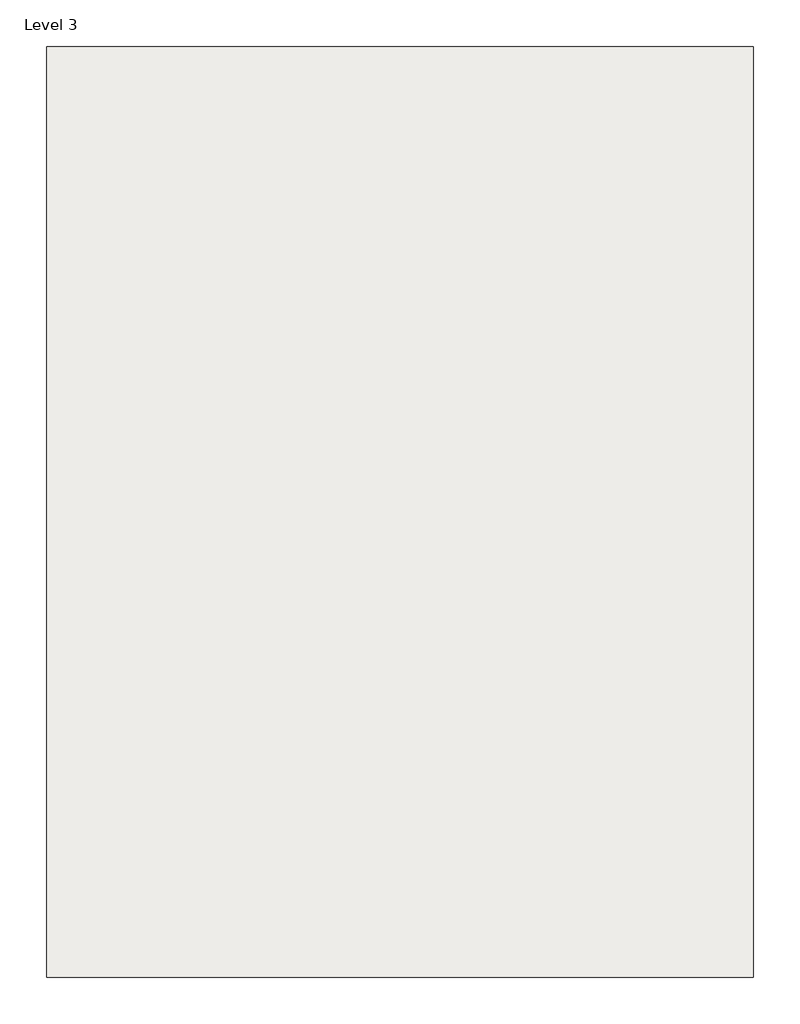
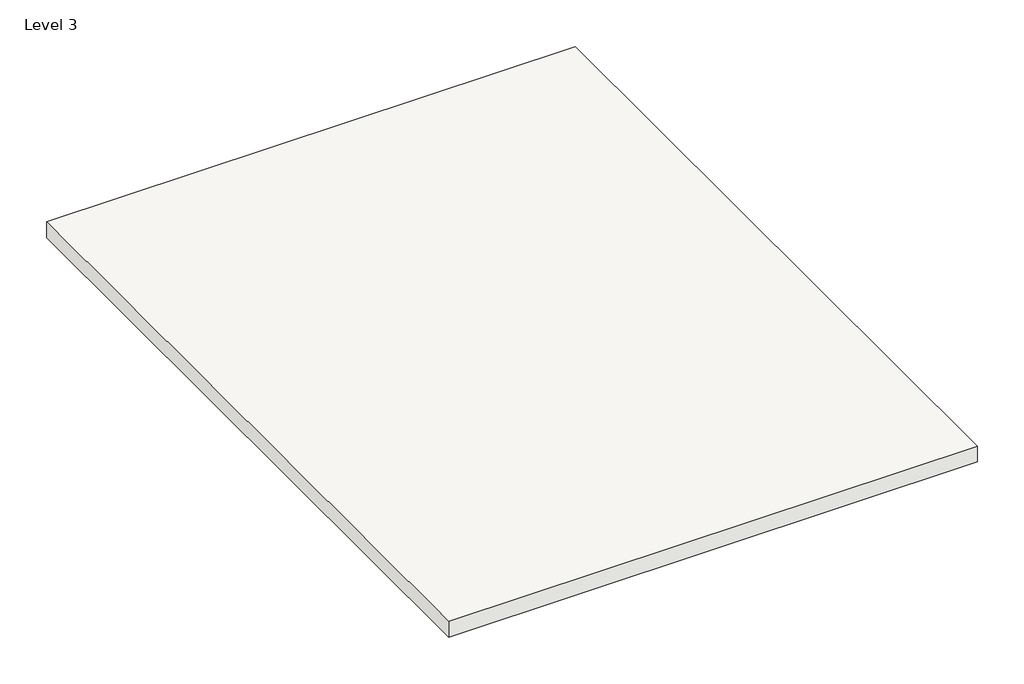
# One storey: 1 roof.
"""IFC4 building model written with IfcOpenShell, lengths in millimetres."""

from ifc_helpers import new_model, si_unit, frame, origin, place, context, project, spatial, polyline, outline, extrude, element, save

model = new_model("IFC4")

# Units and contexts
model_context = context("Model", 3, world=origin())
ifc_project = project(units=[si_unit("LENGTHUNIT", "METRE", prefix="MILLI")], contexts=[model_context])

# Site, building, storey
site = spatial("IfcSite", under=ifc_project)
building = spatial("IfcBuilding", under=site)
storey = spatial("IfcBuildingStorey", under=building, Name="Level 3", Elevation=6096.0)

# Roof
placement = place(None, origin())
element("IfcRoof", 1, ObjectType="Generic - 12\"", at=placement, inside=storey, context=model_context, shape_type="SweptSolid", body=[
    extrude(outline(polyline([(-17178.387855, 181.8231753), (-7577.187855, 181.8231753), (-7577.187855, -12467.3768247), (-17178.387855, -12467.3768247), (-17178.387855, 181.8231753)])), frame((0.0, 0.0, 6096.0), z_axis=(0.0, 0.0, 1.0), x_axis=(1.0, 0.0, 0.0)), (0.0, 0.0, 1.0), 304.8),
])

save(model, "model.ifc")

# Revit data of these elements
# Type "Generic - 12\""
#   Assembly Code = "B1020"
#   Layers, outside or top first: 1' - 0" no material (function 1)
# Element 1 (IfcRoof, "Generic - 12\"")
#   built-in parameter 1001705 = 21 (stored number, unit not read)
#   built-in parameter 1001710 = 33615
#   Phase Created = New Construction
#   Materials on its faces: "Default Roof"
# Materials
#   "Default Roof": colour RGB 88 101 114, transparency 0, Cost = 0
